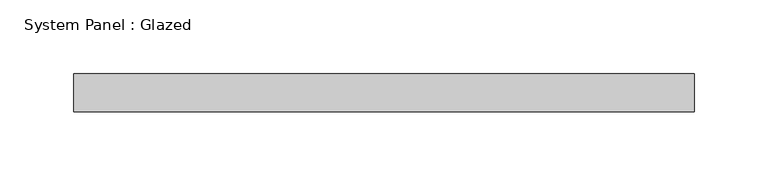
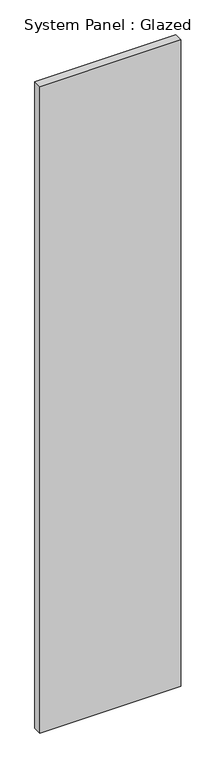
"""IFC4 building model written with IfcOpenShell, lengths in millimetres: plate geometry, System Panel : Glazed."""

from ifc_helpers import new_model, si_unit, origin, origin_with_axes, place, context, project, spatial, polyline, outline, extrude, source, transform, mapped, element, save


def system_panel_glazed_220ba5f3(model_context):
    return source(origin(), model_context, "Body", "SweptSolid", [
        extrude(outline(polyline([(209.6599961, 19.05), (-209.6599961, 19.05), (-209.6599961, 44.45), (209.6599961, 44.45), (209.6599961, 19.05)])), origin_with_axes(), (0.0, 0.0, 1.0), 2032.0),
    ])


if __name__ == "__main__":
    model = new_model("IFC4")
    model_context = context("Model", 3, world=origin())
    ifc_project = project(units=[si_unit("LENGTHUNIT", "METRE", prefix="MILLI")], contexts=[model_context])
    site = spatial("IfcSite", under=ifc_project)
    building = spatial("IfcBuilding", under=site)
    placement = place(None, origin())
    system_panel_glazed_shape = system_panel_glazed_220ba5f3(model_context)
    element("IfcPlate", 1, ObjectType="System Panel : Glazed", at=placement, inside=building, context=model_context, shape_type="MappedRepresentation", body=[
        mapped(system_panel_glazed_shape, transform((0.0, 0.0, 0.0), x_axis=(1.0, 0.0, 0.0), y_axis=(0.0, 1.0, 0.0), z_axis=(0.0, 0.0, 1.0))),
    ])
    save(model, "model.ifc")

# Revit data of these elements
# Type "System Panel : Glazed"
#   Construction Type Id = "GSP4R"
#   Analytic Construction = "1/8 in Pilkington single glazing"
#   Visual Light Transmittance = 0.9
#   Solar Heat Gain Coefficient = 0.86
#   Heat Transfer Coefficient (U) = 1.18115 BTU/(h·ft²·°F)
# Element 1 (IfcPlate, "System Panel : Glazed")
#   Materials on its faces: "Glass"
# Materials
#   "Glass": class "Glass", colour RGB 0 128 192, transparency 0.75, Description = "Soda Lime Glass", Cost = 0
